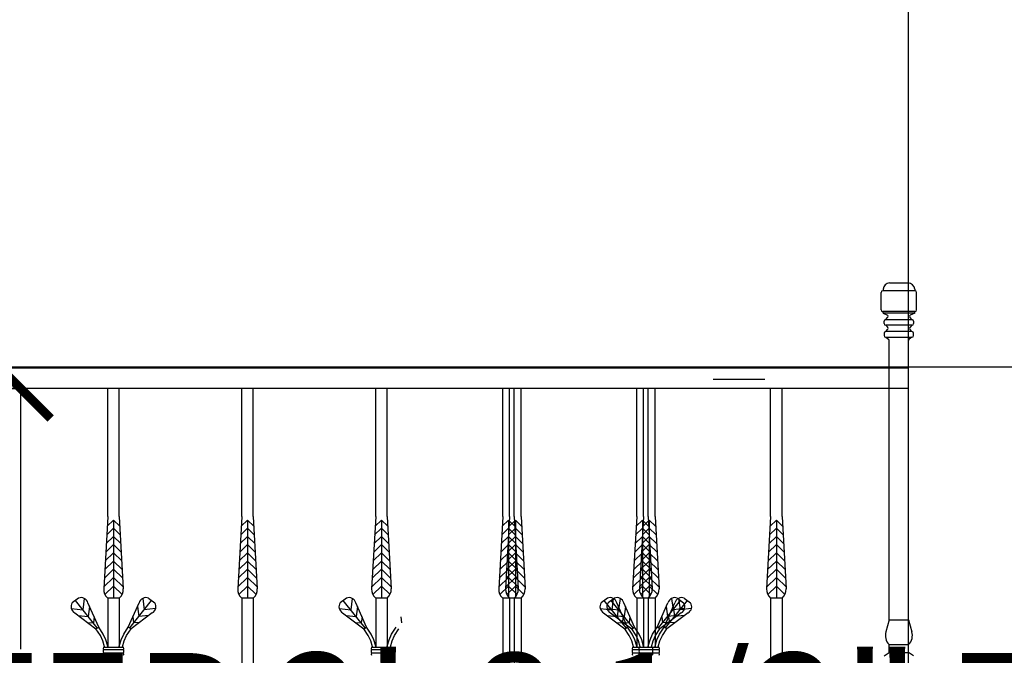
# Model space of a CAD drawing. Units: inches. Extents: x 2278 to 7495, y -71 to 1198.
# Tile 35 of 44: x 5101 to 5150, y 146 to 178. Entities that reach past the tile are written whole.
import ezdxf

# ---------------------------------------------------------------- set-up
doc = ezdxf.new("R2010")
doc.units = ezdxf.units.IN
doc.header["$MEASUREMENT"] = 0
doc.layers.add('A-ANNO-DIMS', color=2, linetype='Continuous', lineweight=18)
doc.layers.add('A-ELEV', color=7, linetype='Continuous', lineweight=25)
doc.styles.get("Standard").update_dxf_attribs({"font": 'arial.ttf'})
doc.dimstyles.get("Standard").update_dxf_attribs({"dimtxt": 6, "dimasz": 3, "dimexe": 0.18, "dimexo": 0.0625, "dimgap": 0.09, "dimtad": 0, "dimtih": 1, "dimtoh": 1, "dimdec": 0, "dimzin": 0, "dimdsep": 46, "dimlunit": 3, "dimtxsty": 'Standard', "dimblk": 'ARCHTICK', "dimcen": 0.09, "dimadec": 0, "dimazin": 0, "dimtfac": 1, "dimtdec": 0, "dimtofl": 0, "dimtmove": 0, "dimatfit": 3, "dimfxl": 1, "dimtolj": 1, "dimtzin": 0, "dimarcsym": 0})

# ---------------------------------------------------------------- blocks, each defined once
blk = doc.blocks.new('BALUSTER-ORNATE-A')
for p, q in [((3.585, 26.003), (3.585, 32.384)), ((4.155, 26.003), (4.155, 32.38)), ((3.585, 26.003), (3.383, 22.393)), ((3.558, 25.516), (3.87, 25.818)), ((3.87, 25.818), (3.87, 21.929)), ((4.182, 25.516), (3.87, 25.818)), ((4.155, 26.003), (4.357, 22.393)), ((3.533, 25.084), (3.87, 25.41)), ((4.207, 25.084), (3.87, 25.41)), ((3.485, 24.221), (3.87, 24.593)), ((3.509, 24.653), (3.87, 25.001)), ((4.231, 24.653), (3.87, 25.001)), ((4.255, 24.221), (3.87, 24.593)), ((3.461, 23.79), (3.87, 24.185)), ((4.279, 23.79), (3.87, 24.185)), ((3.437, 23.358), (3.87, 23.777)), ((4.303, 23.358), (3.87, 23.777)), ((3.413, 22.927), (3.87, 23.369)), ((4.327, 22.927), (3.87, 23.369)), ((3.388, 22.495), (3.87, 22.961)), ((4.352, 22.495), (3.87, 22.961)), ((3.442, 22.106), (3.87, 22.52)), ((4.299, 22.106), (3.87, 22.52)), ((2.128, 21.929), (1.813, 21.699)), ((3.063, 20.442), (1.97, 21.814)), ((2.412, 21.914), (2.339, 21.352)), ((3.131, 20.487), (2.594, 21.696)), ((3.585, 21.929), (3.585, 19.485)), ((4.155, 21.929), (3.585, 21.929)), ((4.155, 21.929), (4.155, 19.485)), ((4.609, 20.487), (5.146, 21.696)), ((4.677, 20.442), (5.77, 21.814)), ((5.328, 21.914), (5.401, 21.352)), ((5.612, 21.929), (5.927, 21.699)), ((1.774, 21.406), (2.339, 21.352)), ((1.936, 21.192), (2.995, 20.398)), ((2.678, 21.507), (2.613, 21.007)), ((5.804, 21.192), (4.745, 20.398)), ((5.062, 21.507), (5.127, 21.007)), ((5.966, 21.406), (5.401, 21.352)), ((2.111, 21.055), (2.613, 21.007)), ((2.562, 20.717), (2.868, 20.688)), ((2.907, 20.992), (2.868, 20.688)), ((4.833, 20.992), (4.872, 20.688)), ((5.178, 20.717), (4.872, 20.688)), ((5.629, 21.055), (5.127, 21.007)), ((2.995, 20.398), (3.131, 20.487)), ((3.217, 20.057), (2.995, 20.398)), ((3.36, 20.135), (3.131, 20.487)), ((3.49, 19.852), (3.36, 20.135)), ((4.25, 19.852), (4.38, 20.135)), ((4.38, 20.135), (4.609, 20.487)), ((4.523, 20.057), (4.745, 20.398)), ((4.745, 20.398), (4.609, 20.487)), ((3.337, 19.795), (3.217, 20.057)), ((3.421, 19.506), (3.337, 19.795)), ((3.585, 19.526), (3.49, 19.852)), ((4.155, 19.526), (4.25, 19.852)), ((4.319, 19.506), (4.403, 19.795)), ((4.403, 19.795), (4.523, 20.057)), ((3.37, 19.485), (4.37, 19.485)), ((3.37, 19.363), (4.37, 19.363)), ((3.37, 19.2), (4.37, 19.2)), ((3.42, 19.485), (3.421, 19.506)), ((3.583, 19.485), (3.585, 19.526)), ((4.157, 19.485), (4.155, 19.526)), ((4.32, 19.485), (4.319, 19.506))]:
    blk.add_line(p, q)
for centre, radius, start, end in [((3.929, 22.355), 0.547, 176.0178, 231.0717), ((3.811, 22.355), 0.547, 308.9283, 3.9822), ((2.111, 21.502), 0.356, 146.575, 240.6788), ((2.253, 21.595), 0.356, 16.4025, 110.5063), ((5.487, 21.595), 0.356, 69.4937, 163.5975), ((5.629, 21.502), 0.356, 299.3212, 33.425), ((3.475, 19.424), 0.121, 149.7768, 210.2232), ((3.563, 19.281), 0.209, 157.1017, 202.8983), ((3.475, 19.139), 0.121, 149.7768, 210.2232), ((4.265, 19.424), 0.121, 329.7768, 30.2232), ((4.177, 19.281), 0.209, 337.1017, 22.8983), ((4.265, 19.139), 0.121, 329.7768, 30.2232)]:
    blk.add_arc(centre, radius, start, end)
blk = doc.blocks.new('BALUSTER-ORNATE-B')
for p, q in [((3.585, 26.003), (3.585, 32.384)), ((4.155, 26.003), (4.155, 32.38)), ((3.585, 26.003), (3.383, 22.393)), ((3.558, 25.516), (3.87, 25.818)), ((3.87, 25.818), (3.87, 21.929)), ((4.183, 25.516), (3.87, 25.818)), ((4.155, 26.003), (4.358, 22.393)), ((3.534, 25.084), (3.87, 25.41)), ((4.207, 25.084), (3.87, 25.41)), ((3.485, 24.221), (3.87, 24.593)), ((3.51, 24.653), (3.87, 25.001)), ((4.231, 24.653), (3.87, 25.001)), ((4.255, 24.221), (3.87, 24.593)), ((3.461, 23.79), (3.87, 24.185)), ((4.279, 23.79), (3.87, 24.185)), ((3.437, 23.358), (3.87, 23.777)), ((4.304, 23.358), (3.87, 23.777)), ((3.413, 22.927), (3.87, 23.369)), ((4.328, 22.927), (3.87, 23.369)), ((3.389, 22.495), (3.87, 22.961)), ((4.352, 22.495), (3.87, 22.961)), ((3.442, 22.106), (3.87, 22.52)), ((4.299, 22.106), (3.87, 22.52)), ((2.128, 21.929), (1.814, 21.699)), ((3.063, 20.442), (1.971, 21.814)), ((2.412, 21.914), (2.339, 21.352)), ((3.132, 20.487), (2.595, 21.696)), ((3.585, 21.929), (3.585, 19.485)), ((4.155, 21.929), (3.585, 21.929)), ((4.155, 21.929), (4.155, 19.485)), ((1.774, 21.406), (2.339, 21.352)), ((1.936, 21.192), (2.995, 20.398)), ((2.679, 21.507), (2.614, 21.007)), ((2.112, 21.055), (2.614, 21.007)), ((2.563, 20.717), (2.868, 20.688)), ((2.907, 20.992), (2.868, 20.688)), ((4.833, 20.992), (4.873, 20.688)), ((2.995, 20.398), (3.132, 20.487)), ((3.217, 20.057), (2.995, 20.398)), ((3.36, 20.135), (3.132, 20.487)), ((3.49, 19.852), (3.36, 20.135)), ((4.251, 19.852), (4.381, 20.135)), ((4.381, 20.135), (4.609, 20.487)), ((4.524, 20.057), (4.746, 20.398)), ((3.337, 19.795), (3.217, 20.057)), ((3.421, 19.506), (3.337, 19.795)), ((3.585, 19.526), (3.49, 19.852)), ((4.155, 19.526), (4.251, 19.852)), ((4.319, 19.506), (4.404, 19.795)), ((4.404, 19.795), (4.524, 20.057)), ((3.37, 19.485), (4.37, 19.485)), ((3.37, 19.363), (4.37, 19.363)), ((3.37, 19.2), (4.37, 19.2)), ((3.42, 19.485), (3.421, 19.506)), ((3.583, 19.485), (3.585, 19.526)), ((4.157, 19.485), (4.155, 19.526)), ((4.32, 19.485), (4.319, 19.506))]:
    blk.add_line(p, q)
for centre, radius, start, end in [((3.929, 22.355), 0.547, 176.0178, 231.0717), ((3.811, 22.355), 0.547, 308.9283, 3.9822), ((2.111, 21.502), 0.356, 146.575, 240.6788), ((2.253, 21.595), 0.356, 16.4025, 110.5063), ((3.475, 19.424), 0.121, 149.7768, 210.2232), ((3.563, 19.281), 0.209, 157.1017, 202.8983), ((3.475, 19.139), 0.121, 149.7768, 210.2232), ((4.265, 19.424), 0.121, 329.7768, 30.2232), ((4.177, 19.281), 0.209, 337.1017, 22.8983), ((4.265, 19.139), 0.121, 329.7768, 30.2232)]:
    blk.add_arc(centre, radius, start, end)
blk = doc.blocks.new('RAIL-BAR-C')
for p, q in [((0.203, 26.003), (0.203, 32.38)), ((0.773, 32.38), (0.203, 32.38)), ((0.773, 26.003), (0.773, 32.38)), ((0.203, 26.003), (0, 22.393)), ((0.175, 25.516), (0.488, 25.818)), ((0.488, 25.818), (0.488, 21.929)), ((0.8, 25.516), (0.488, 25.818)), ((0.773, 26.003), (0.975, 22.393)), ((0.151, 25.084), (0.488, 25.41)), ((0.824, 25.084), (0.488, 25.41)), ((0.103, 24.221), (0.488, 24.593)), ((0.127, 24.653), (0.488, 25.001)), ((0.848, 24.653), (0.488, 25.001)), ((0.873, 24.221), (0.488, 24.593)), ((0.079, 23.79), (0.488, 24.185)), ((0.897, 23.79), (0.488, 24.185)), ((0.054, 23.358), (0.488, 23.777)), ((0.921, 23.358), (0.488, 23.777)), ((0.03, 22.927), (0.488, 23.369)), ((0.945, 22.927), (0.488, 23.369)), ((0.006, 22.495), (0.488, 22.961)), ((0.969, 22.495), (0.488, 22.961)), ((0.059, 22.106), (0.488, 22.52)), ((0.916, 22.106), (0.488, 22.52)), ((0.203, 21.929), (0.203, 7.128)), ((0.773, 21.929), (0.203, 21.929)), ((0.773, 21.929), (0.773, 7.128))]:
    blk.add_line(p, q)
for centre, start, end in [((0.547, 22.355), 176.0178, 231.0717), ((0.429, 22.355), 308.9283, 3.9822)]:
    blk.add_arc(centre, 0.547, start, end)
blk = doc.blocks.new('_ArchTick')
at = {"color": 0, "linetype": 'ByBlock', "const_width": 0.15}
blk.add_lwpolyline([(-0.5, -0.5), (0.5, 0.5)], dxfattribs=at)
blk = doc.blocks.new('*D59')
at = {"layer": 'A-ANNO-DIMS', "color": 0, "lineweight": -2, "transparency": 16777216}
for p, q in [((5096.589, 159.183), (5101.564, 159.183)), ((5101.384, 159.183), (5101.384, 146.185)), ((5101.384, 126.799), (5101.384, 139.796)), ((5096.589, 126.799), (5101.564, 126.799))]:
    blk.add_line(p, q, dxfattribs=at)
at = {"layer": 'Defpoints', "color": 0, "transparency": 16777216}
for p in [(5096.527, 159.183), (5101.384, 159.183), (5096.527, 126.799)]:
    blk.add_point(p, dxfattribs=at)
at = {"layer": 'A-ANNO-DIMS', "color": 0, "lineweight": -2, "transparency": 16777216, "xscale": 3, "yscale": 3, "zscale": 3}
for p, rotation in [((5101.384, 159.183), 90), ((5101.384, 126.799), 270)]:
    blk.add_blockref('_ArchTick', p, dxfattribs=dict(at, rotation=rotation))
at = {"layer": 'A-ANNO-DIMS', "color": 0, "transparency": 16777216, "insert": (5101.384, 142.991), "char_height": 6, "attachment_point": 5}
blk.add_mtext('\\A1;ORNATE BALUSTER 2\'-8 1/2" TYP.', dxfattribs=at)
blk = doc.blocks.new('*D123')
at = {"layer": 'A-ANNO-DIMS', "color": 0, "lineweight": -2, "transparency": 16777216}
for p, q in [((4736.95, 340.157), (4736.95, -23.427)), ((5145.676, -1.81), (5145.676, -23.427)), ((4736.95, -23.247), (4923.929, -23.247)), ((5145.676, -23.247), (4958.697, -23.247))]:
    blk.add_line(p, q, dxfattribs=at)
at = {"layer": 'Defpoints', "color": 0, "transparency": 16777216}
for p in [(4736.95, 340.219), (5145.676, -1.747), (5145.676, -23.247)]:
    blk.add_point(p, dxfattribs=at)
at = {"layer": 'A-ANNO-DIMS', "color": 0, "lineweight": -2, "transparency": 16777216, "xscale": 3, "yscale": 3, "zscale": 3, "rotation": 180}
blk.add_blockref('_ArchTick', (4736.95, -23.247), dxfattribs=at)
at = {"layer": 'A-ANNO-DIMS', "color": 0, "lineweight": -2, "transparency": 16777216, "xscale": 3, "yscale": 3, "zscale": 3}
blk.add_blockref('_ArchTick', (5145.676, -23.247), dxfattribs=at)
at = {"layer": 'A-ANNO-DIMS', "color": 0, "transparency": 16777216, "insert": (4941.313, -23.247), "char_height": 6, "attachment_point": 5}
blk.add_mtext('\\A1;34\'-0 1/2"', dxfattribs=at)
blk = doc.blocks.new('*D131')
at = {"layer": 'A-ANNO-DIMS', "color": 0, "lineweight": -2, "transparency": 16777216}
for p, q in [((5096.176, 99.315), (5096.176, 361.899)), ((5096.176, 361.719), (5105.75, 361.719)), ((5145.676, 361.719), (5136.102, 361.719)), ((5145.676, 118.315), (5145.676, 361.899))]:
    blk.add_line(p, q, dxfattribs=at)
at = {"layer": 'Defpoints', "color": 0, "transparency": 16777216}
for p in [(5145.676, 361.719), (5145.676, 118.253), (5096.176, 99.253)]:
    blk.add_point(p, dxfattribs=at)
at = {"layer": 'A-ANNO-DIMS', "color": 0, "lineweight": -2, "transparency": 16777216, "xscale": 3, "yscale": 3, "zscale": 3, "rotation": 180}
blk.add_blockref('_ArchTick', (5096.176, 361.719), dxfattribs=at)
at = {"layer": 'A-ANNO-DIMS', "color": 0, "lineweight": -2, "transparency": 16777216, "xscale": 3, "yscale": 3, "zscale": 3}
blk.add_blockref('_ArchTick', (5145.676, 361.719), dxfattribs=at)
at = {"layer": 'A-ANNO-DIMS', "color": 0, "transparency": 16777216, "insert": (5120.926, 361.719), "char_height": 6, "attachment_point": 5}
blk.add_mtext('\\A1;4\'-1 1/2"', dxfattribs=at)
blk = doc.blocks.new('*D139')
at = {"layer": 'A-ANNO-DIMS', "color": 0, "lineweight": -2, "transparency": 16777216}
for p, q in [((5092.239, 160.253), (5167.754, 160.253)), ((5167.574, 160.253), (5167.574, 142.408)), ((5167.574, 118.253), (5167.574, 136.097)), ((5145.739, 118.253), (5167.754, 118.253))]:
    blk.add_line(p, q, dxfattribs=at)
at = {"layer": 'Defpoints', "color": 0, "transparency": 16777216}
for p in [(5092.176, 160.253), (5167.574, 160.253), (5145.676, 118.253)]:
    blk.add_point(p, dxfattribs=at)
at = {"layer": 'A-ANNO-DIMS', "color": 0, "lineweight": -2, "transparency": 16777216, "xscale": 3, "yscale": 3, "zscale": 3}
for p, rotation in [((5167.574, 160.253), 90), ((5167.574, 118.253), 270)]:
    blk.add_blockref('_ArchTick', p, dxfattribs=dict(at, rotation=rotation))
at = {"layer": 'A-ANNO-DIMS', "color": 0, "transparency": 16777216, "insert": (5167.574, 139.253), "char_height": 6, "attachment_point": 5}
blk.add_mtext('\\A1;3\'-6"', dxfattribs=at)
blk = doc.blocks.new('*D140')
at = {"layer": 'A-ANNO-DIMS', "color": 0, "lineweight": -2, "transparency": 16777216}
for p, q in [((5096.239, 225.253), (5167.754, 225.253)), ((5167.574, 225.253), (5167.574, 195.894)), ((5167.574, 160.253), (5167.574, 189.612)), ((5092.239, 160.253), (5167.754, 160.253))]:
    blk.add_line(p, q, dxfattribs=at)
at = {"layer": 'Defpoints', "color": 0, "transparency": 16777216}
for p in [(5096.176, 225.253), (5167.574, 225.253), (5092.176, 160.253)]:
    blk.add_point(p, dxfattribs=at)
at = {"layer": 'A-ANNO-DIMS', "color": 0, "lineweight": -2, "transparency": 16777216, "xscale": 3, "yscale": 3, "zscale": 3}
for p, rotation in [((5167.574, 225.253), 90), ((5167.574, 160.253), 270)]:
    blk.add_blockref('_ArchTick', p, dxfattribs=dict(at, rotation=rotation))
at = {"layer": 'A-ANNO-DIMS', "color": 0, "transparency": 16777216, "insert": (5167.574, 192.753), "char_height": 6, "attachment_point": 5}
blk.add_mtext('\\A1;5\'-5"', dxfattribs=at)
blk = doc.blocks.new('*D144')
at = {"layer": 'A-ANNO-DIMS', "color": 0, "lineweight": -2, "transparency": 16777216}
for p, q in [((5145.739, 244.253), (5167.754, 244.253)), ((5167.574, 244.253), (5167.574, 184.406)), ((5167.574, 118.253), (5167.574, 178.099)), ((5145.739, 118.253), (5167.754, 118.253))]:
    blk.add_line(p, q, dxfattribs=at)
at = {"layer": 'Defpoints', "color": 0, "transparency": 16777216}
for p in [(5145.676, 244.253), (5167.574, 244.253), (5145.676, 118.253)]:
    blk.add_point(p, dxfattribs=at)
at = {"layer": 'A-ANNO-DIMS', "color": 0, "lineweight": -2, "transparency": 16777216, "xscale": 3, "yscale": 3, "zscale": 3}
for p, rotation in [((5167.574, 244.253), 90), ((5167.574, 118.253), 270)]:
    blk.add_blockref('_ArchTick', p, dxfattribs=dict(at, rotation=rotation))
at = {"layer": 'A-ANNO-DIMS', "color": 0, "transparency": 16777216, "insert": (5167.574, 181.253), "char_height": 6, "attachment_point": 5}
blk.add_mtext('\\A1;10\'-6"', dxfattribs=at)

msp = doc.modelspace()

# ---------------------------------------------------------------- linework, layer by layer
at = {"layer": 'A-ELEV'}
for p, q in [((5145.676, 164.446), (5145.676, 250.254)), ((5145.992, 164.046), (5144.383, 164.046)), ((5144.397, 164.122), (5144.397, 164.046)), ((5144.726, 164.449), (5145.648, 164.449)), ((5145.978, 164.122), (5145.978, 164.046)), ((5144.301, 163.092), (5144.301, 163.965)), ((5146.074, 163.092), (5146.074, 163.965)), ((5145.992, 163.01), (5144.383, 163.01)), ((5144.397, 162.934), (5144.397, 163.01)), ((5144.397, 162.934), (5144.622, 162.837)), ((5145.978, 162.934), (5144.397, 162.934)), ((5144.536, 162.615), (5144.622, 162.711)), ((5144.536, 162.615), (5145.839, 162.615)), ((5145.978, 162.934), (5145.753, 162.837)), ((5145.839, 162.615), (5145.753, 162.711)), ((5145.978, 162.934), (5145.978, 163.01)), ((5144.454, 162.416), (5144.454, 162.533)), ((5144.536, 162.334), (5144.622, 162.238)), ((5145.839, 162.334), (5144.536, 162.334)), ((5144.536, 162.015), (5144.622, 162.112)), ((5145.839, 162.334), (5145.753, 162.238)), ((5145.839, 162.015), (5145.753, 162.112)), ((5145.921, 162.533), (5145.921, 162.416)), ((5144.454, 161.934), (5144.454, 161.816)), ((5145.839, 162.015), (5144.536, 162.015)), ((5144.536, 161.735), (5144.669, 161.64)), ((5144.536, 161.735), (5145.839, 161.735)), ((5144.699, 147.642), (5144.699, 161.577)), ((5145.676, -1.747), (5145.676, 161.577)), ((5145.676, 147.642), (5145.676, 161.577)), ((5145.839, 161.735), (5145.706, 161.64)), ((5145.921, 161.816), (5145.921, 161.934)), ((5145.676, 160.198), (5066.016, 160.198)), ((5138.507, 159.631), (5135.918, 159.631)), ((5145.676, 159.179), (5066.016, 159.179)), ((5125.431, 152.802), (5125.431, 159.179)), ((5125.775, 152.802), (5125.775, 159.179)), ((5126.001, 152.802), (5126.001, 159.179)), ((5126.345, 152.802), (5126.345, 159.179)), ((5132.111, 152.802), (5132.111, 159.183)), ((5132.455, 152.802), (5132.455, 159.183)), ((5132.682, 152.802), (5132.682, 159.179)), ((5133.026, 152.802), (5133.026, 159.179)), ((5138.792, 152.802), (5138.792, 159.179)), ((5139.362, 152.802), (5139.362, 159.179)), ((5125.431, 152.802), (5125.229, 149.192)), ((5125.775, 152.802), (5125.573, 149.192)), ((5126.001, 152.802), (5126.203, 149.192)), ((5126.345, 152.802), (5126.547, 149.192)), ((5132.111, 152.802), (5131.909, 149.192)), ((5132.455, 152.802), (5132.253, 149.192)), ((5132.682, 152.802), (5132.884, 149.192)), ((5133.026, 152.802), (5133.228, 149.192)), ((5138.792, 152.802), (5138.59, 149.192)), ((5139.362, 152.802), (5139.564, 149.192)), ((5125.404, 152.315), (5125.716, 152.617)), ((5125.716, 152.617), (5125.716, 148.728)), ((5126.028, 152.315), (5125.716, 152.617)), ((5125.747, 152.315), (5126.06, 152.617)), ((5126.06, 152.617), (5126.06, 148.728)), ((5126.372, 152.315), (5126.06, 152.617)), ((5132.084, 152.315), (5132.397, 152.617)), ((5132.397, 152.617), (5132.397, 148.728)), ((5132.709, 152.315), (5132.397, 152.617)), ((5132.428, 152.315), (5132.74, 152.617)), ((5132.74, 152.617), (5132.74, 148.728)), ((5133.053, 152.315), (5132.74, 152.617)), ((5138.765, 152.315), (5139.077, 152.617)), ((5139.077, 152.617), (5139.077, 148.728)), ((5139.39, 152.315), (5139.077, 152.617)), ((5125.355, 151.452), (5125.716, 151.8)), ((5125.379, 151.883), (5125.716, 152.209)), ((5125.699, 151.452), (5126.06, 151.8)), ((5126.053, 151.883), (5125.716, 152.209)), ((5126.077, 151.452), (5125.716, 151.8)), ((5125.723, 151.883), (5126.06, 152.209)), ((5126.396, 151.883), (5126.06, 152.209)), ((5126.421, 151.452), (5126.06, 151.8)), ((5132.036, 151.452), (5132.397, 151.8)), ((5132.06, 151.883), (5132.397, 152.209)), ((5132.38, 151.452), (5132.74, 151.8)), ((5132.733, 151.883), (5132.397, 152.209)), ((5132.757, 151.452), (5132.397, 151.8)), ((5132.404, 151.883), (5132.74, 152.209)), ((5133.077, 151.883), (5132.74, 152.209)), ((5133.101, 151.452), (5132.74, 151.8)), ((5138.716, 151.452), (5139.077, 151.8)), ((5138.741, 151.883), (5139.077, 152.209)), ((5139.414, 151.883), (5139.077, 152.209)), ((5139.438, 151.452), (5139.077, 151.8)), ((5125.331, 151.02), (5125.716, 151.392)), ((5125.675, 151.02), (5126.06, 151.392)), ((5126.101, 151.02), (5125.716, 151.392)), ((5126.445, 151.02), (5126.06, 151.392)), ((5132.012, 151.02), (5132.397, 151.392)), ((5132.356, 151.02), (5132.74, 151.392)), ((5132.781, 151.02), (5132.397, 151.392)), ((5133.125, 151.02), (5132.74, 151.392)), ((5138.692, 151.02), (5139.077, 151.392)), ((5139.462, 151.02), (5139.077, 151.392)), ((5125.307, 150.589), (5125.716, 150.984)), ((5125.651, 150.589), (5126.06, 150.984)), ((5126.125, 150.589), (5125.716, 150.984)), ((5126.469, 150.589), (5126.06, 150.984)), ((5131.987, 150.589), (5132.397, 150.984)), ((5132.331, 150.589), (5132.74, 150.984)), ((5132.806, 150.589), (5132.397, 150.984)), ((5133.15, 150.589), (5132.74, 150.984)), ((5138.668, 150.589), (5139.077, 150.984)), ((5139.486, 150.589), (5139.077, 150.984)), ((5125.283, 150.157), (5125.716, 150.576)), ((5125.627, 150.157), (5126.06, 150.576)), ((5126.149, 150.157), (5125.716, 150.576)), ((5126.493, 150.157), (5126.06, 150.576)), ((5131.963, 150.157), (5132.397, 150.576)), ((5132.307, 150.157), (5132.74, 150.576)), ((5132.83, 150.157), (5132.397, 150.576)), ((5133.174, 150.157), (5132.74, 150.576)), ((5138.644, 150.157), (5139.077, 150.576)), ((5139.51, 150.157), (5139.077, 150.576)), ((5125.259, 149.726), (5125.716, 150.168)), ((5125.602, 149.726), (5126.06, 150.168)), ((5126.173, 149.726), (5125.716, 150.168)), ((5126.517, 149.726), (5126.06, 150.168)), ((5131.939, 149.726), (5132.397, 150.168)), ((5132.283, 149.726), (5132.74, 150.168)), ((5132.854, 149.726), (5132.397, 150.168)), ((5133.198, 149.726), (5132.74, 150.168)), ((5138.62, 149.726), (5139.077, 150.168)), ((5139.535, 149.726), (5139.077, 150.168)), ((5125.234, 149.294), (5125.716, 149.76)), ((5125.287, 148.905), (5125.716, 149.319)), ((5125.578, 149.294), (5126.06, 149.76)), ((5125.631, 148.905), (5126.06, 149.319)), ((5126.198, 149.294), (5125.716, 149.76)), ((5126.144, 148.905), (5125.716, 149.319)), ((5126.541, 149.294), (5126.06, 149.76)), ((5126.488, 148.905), (5126.06, 149.319)), ((5131.915, 149.294), (5132.397, 149.76)), ((5131.968, 148.905), (5132.397, 149.319)), ((5132.259, 149.294), (5132.74, 149.76)), ((5132.312, 148.905), (5132.74, 149.319)), ((5132.878, 149.294), (5132.397, 149.76)), ((5132.825, 148.905), (5132.397, 149.319)), ((5133.222, 149.294), (5132.74, 149.76)), ((5133.169, 148.905), (5132.74, 149.319)), ((5138.596, 149.294), (5139.077, 149.76)), ((5138.649, 148.905), (5139.077, 149.319)), ((5139.559, 149.294), (5139.077, 149.76)), ((5139.506, 148.905), (5139.077, 149.319)), ((5125.431, 148.728), (5125.431, 133.927)), ((5126.001, 148.728), (5125.431, 148.728)), ((5125.775, 148.728), (5125.775, 133.927)), ((5126.345, 148.728), (5125.775, 148.728)), ((5126.001, 148.728), (5126.001, 133.927)), ((5126.345, 148.728), (5126.345, 133.927)), ((5130.654, 148.728), (5130.34, 148.498)), ((5131.59, 147.241), (5130.497, 148.613)), ((5130.998, 148.728), (5130.684, 148.498)), ((5131.934, 147.241), (5130.841, 148.613)), ((5130.938, 148.713), (5130.865, 148.151)), ((5131.658, 147.286), (5131.121, 148.495)), ((5131.282, 148.713), (5131.209, 148.151)), ((5132.002, 147.286), (5131.465, 148.495)), ((5132.111, 148.728), (5132.111, 146.284)), ((5132.682, 148.728), (5132.111, 148.728)), ((5132.455, 148.728), (5132.455, 146.284)), ((5133.026, 148.728), (5132.455, 148.728)), ((5132.682, 148.728), (5132.682, 146.284)), ((5133.026, 148.728), (5133.026, 146.284)), ((5133.135, 147.286), (5133.672, 148.495)), ((5133.203, 147.241), (5134.296, 148.613)), ((5133.479, 147.286), (5134.016, 148.495)), ((5133.547, 147.241), (5134.64, 148.613)), ((5133.855, 148.713), (5133.928, 148.151)), ((5134.139, 148.728), (5134.453, 148.498)), ((5134.199, 148.713), (5134.272, 148.151)), ((5134.483, 148.728), (5134.797, 148.498)), ((5138.792, 148.728), (5138.792, 133.927)), ((5139.362, 148.728), (5138.792, 148.728)), ((5139.362, 148.728), (5139.362, 133.927)), ((5130.301, 148.205), (5130.865, 148.151)), ((5130.463, 147.991), (5131.521, 147.197)), ((5130.638, 147.854), (5131.14, 147.806)), ((5130.645, 148.205), (5131.209, 148.151)), ((5130.807, 147.991), (5131.865, 147.197)), ((5130.982, 147.854), (5131.484, 147.806)), ((5131.205, 148.306), (5131.14, 147.806)), ((5131.549, 148.306), (5131.484, 147.806)), ((5134.33, 147.991), (5133.272, 147.197)), ((5133.588, 148.306), (5133.653, 147.806)), ((5134.674, 147.991), (5133.616, 147.197)), ((5134.155, 147.854), (5133.653, 147.806)), ((5134.493, 148.205), (5133.928, 148.151)), ((5133.932, 148.306), (5133.997, 147.806)), ((5134.499, 147.854), (5133.997, 147.806)), ((5134.836, 148.205), (5134.272, 148.151)), ((5131.089, 147.516), (5131.394, 147.487)), ((5131.434, 147.791), (5131.394, 147.487)), ((5131.433, 147.516), (5131.738, 147.487)), ((5131.778, 147.791), (5131.738, 147.487)), ((5133.359, 147.791), (5133.399, 147.487)), ((5133.704, 147.516), (5133.399, 147.487)), ((5133.703, 147.791), (5133.743, 147.487)), ((5134.048, 147.516), (5133.743, 147.487)), ((5144.699, 147.642), (5144.546, 147.049)), ((5144.699, 147.642), (5145.676, 147.642)), ((5145.676, 147.642), (5145.829, 147.049)), ((5131.521, 147.197), (5131.658, 147.286)), ((5131.743, 146.856), (5131.521, 147.197)), ((5131.886, 146.934), (5131.658, 147.286)), ((5131.863, 146.594), (5131.743, 146.856)), ((5131.865, 147.197), (5132.002, 147.286)), ((5132.087, 146.856), (5131.865, 147.197)), ((5132.016, 146.651), (5131.886, 146.934)), ((5132.23, 146.934), (5132.002, 147.286)), ((5132.207, 146.594), (5132.087, 146.856)), ((5132.36, 146.651), (5132.23, 146.934)), ((5132.777, 146.651), (5132.907, 146.934)), ((5132.907, 146.934), (5133.135, 147.286)), ((5132.93, 146.594), (5133.05, 146.856)), ((5133.05, 146.856), (5133.272, 147.197)), ((5133.121, 146.651), (5133.251, 146.934)), ((5133.272, 147.197), (5133.135, 147.286)), ((5133.251, 146.934), (5133.479, 147.286)), ((5133.274, 146.594), (5133.394, 146.856)), ((5133.394, 146.856), (5133.616, 147.197)), ((5133.616, 147.197), (5133.479, 147.286)), ((5131.947, 146.305), (5131.863, 146.594)), ((5132.111, 146.325), (5132.016, 146.651)), ((5132.291, 146.305), (5132.207, 146.594)), ((5132.455, 146.325), (5132.36, 146.651)), ((5132.682, 146.325), (5132.777, 146.651)), ((5132.846, 146.305), (5132.93, 146.594)), ((5133.026, 146.325), (5133.121, 146.651)), ((5133.19, 146.305), (5133.274, 146.594)), ((5144.699, 146.42), (5145.676, 146.42)), ((5144.699, 146.012), (5144.699, 146.42)), ((5145.676, 146.012), (5145.676, 146.42)), ((5131.897, 146.284), (5132.897, 146.284)), ((5131.897, 146.162), (5132.897, 146.162)), ((5131.897, 145.999), (5132.897, 145.999)), ((5131.947, 146.284), (5131.947, 146.305)), ((5132.11, 146.284), (5132.111, 146.325)), ((5132.24, 146.284), (5133.241, 146.284)), ((5132.24, 146.162), (5133.241, 146.162)), ((5132.24, 145.999), (5133.241, 145.999)), ((5132.29, 146.284), (5132.291, 146.305)), ((5132.454, 146.284), (5132.455, 146.325)), ((5132.684, 146.284), (5132.682, 146.325)), ((5132.847, 146.284), (5132.846, 146.305)), ((5133.027, 146.284), (5133.026, 146.325)), ((5133.191, 146.284), (5133.19, 146.305)), ((5144.454, 145.849), (5144.699, 146.012)), ((5144.699, 146.012), (5145.676, 146.012)), ((5145.921, 145.849), (5145.676, 146.012))]:
    msp.add_line(p, q, dxfattribs=at)
for centre, radius, start, end in [((5144.383, 163.965), 0.0815, 90, 180), ((5144.749, 164.097), 0.352, 93.6206, 175.8919), ((5145.626, 164.097), 0.352, 4.1081, 86.3794), ((5145.992, 163.965), 0.0815, 0, 90), ((5144.383, 163.092), 0.0815, 180, 270), ((5145.992, 163.092), 0.0815, 270, 0), ((5144.536, 162.533), 0.0815, 90, 180), ((5144.57, 162.774), 0.0815, 309.328, 50.672), ((5145.805, 162.774), 0.0815, 129.328, 230.672), ((5145.839, 162.533), 0.0815, 0, 90), ((5144.536, 162.416), 0.0815, 180, 270), ((5144.57, 162.175), 0.0815, 309.328, 50.672), ((5145.805, 162.175), 0.0815, 129.328, 230.672), ((5145.839, 162.416), 0.0815, 270, 360), ((5144.536, 161.934), 0.0815, 90, 180), ((5144.536, 161.816), 0.0815, 180, 270), ((5144.617, 161.577), 0.0815, 0, 50.672), ((5145.758, 161.577), 0.0815, 129.328, 180), ((5145.839, 161.934), 0.0815, 0, 90), ((5145.839, 161.816), 0.0815, 270, 360), ((5125.775, 149.154), 0.547, 176.0178, 231.0717), ((5126.119, 149.154), 0.547, 176.0178, 231.0717), ((5125.657, 149.154), 0.547, 308.9283, 3.9822), ((5126.001, 149.154), 0.547, 308.9283, 3.9822), ((5132.455, 149.154), 0.547, 176.0178, 231.0717), ((5132.799, 149.154), 0.547, 176.0178, 231.0717), ((5132.338, 149.154), 0.547, 308.9283, 3.9822), ((5132.682, 149.154), 0.547, 308.9283, 3.9822), ((5139.136, 149.154), 0.547, 176.0178, 231.0717), ((5139.018, 149.154), 0.547, 308.9283, 3.9822), ((5130.637, 148.301), 0.356, 146.575, 240.6788), ((5130.981, 148.301), 0.356, 146.575, 240.6788), ((5130.779, 148.394), 0.356, 16.4025, 110.5063), ((5131.123, 148.394), 0.356, 16.4025, 110.5063), ((5134.014, 148.394), 0.356, 69.4937, 163.5975), ((5134.358, 148.394), 0.356, 69.4937, 163.5975), ((5134.156, 148.301), 0.356, 299.3212, 33.425), ((5134.5, 148.301), 0.356, 299.3212, 33.425), ((5145.122, 146.856), 0.608, 161.4732, 225.8681), ((5145.253, 146.856), 0.608, 314.1319, 18.5268), ((5132.001, 146.223), 0.121, 149.7768, 210.2232), ((5132.089, 146.08), 0.209, 157.1017, 202.8983), ((5132.001, 145.938), 0.121, 149.7768, 210.2232), ((5132.345, 146.223), 0.121, 149.7768, 210.2232), ((5132.433, 146.08), 0.209, 157.1017, 202.8983), ((5132.345, 145.938), 0.121, 149.7768, 210.2232), ((5132.792, 146.223), 0.121, 329.7768, 30.2232), ((5132.704, 146.08), 0.209, 337.1017, 22.8983), ((5132.792, 145.938), 0.121, 329.7768, 30.2232), ((5133.136, 146.223), 0.121, 329.7768, 30.2232), ((5133.048, 146.08), 0.209, 337.1017, 22.8983), ((5133.136, 145.938), 0.121, 329.7768, 30.2232)]:
    msp.add_arc(centre, radius, start, end, dxfattribs=at)

# ---------------------------------------------------------------- block references
for name, p in [('BALUSTER-ORNATE-A', (5102.148, 126.799)), ('RAIL-BAR-C', (5112.211, 126.799)), ('BALUSTER-ORNATE-B', (5115.509, 126.799))]:
    msp.add_blockref(name, p, dxfattribs=at)

# ---------------------------------------------------------------- dimensions: what is measured, and where the dimension line sits
at = {"layer": 'A-ANNO-DIMS'}
for base, p1, p2, picture, middle in [((5145.676, 361.719), (5096.176, 99.253), (5145.676, 118.253), '*D131', (5120.926, 361.719)), ((5145.676, -23.247), (4736.95, 340.219), (5145.676, -1.747), '*D123', (4941.313, -23.247))]:
    dim = msp.add_linear_dim(base=base, p1=p1, p2=p2, dimstyle='Standard', override={"dimdec": 1, "dimlfac": 1, "dimrnd": 0, "dimzin": 1, "dimdsep": 46, "dimlunit": 4, "dimfrac": 2}, dxfattribs=at)
    dim.commit()
    dim.dimension.update_dxf_attribs({"geometry": picture, "text_midpoint": middle})
for base, p1, p2, picture, middle in [((5167.574, 244.253), (5145.676, 118.253), (5145.676, 244.253), '*D144', (5167.574, 181.253)), ((5167.574, 225.253), (5092.176, 160.253), (5096.176, 225.253), '*D140', (5167.574, 192.753)), ((5167.574, 160.253), (5145.676, 118.253), (5092.176, 160.253), '*D139', (5167.574, 139.253))]:
    dim = msp.add_linear_dim(base=base, p1=p1, p2=p2, angle=90, dimstyle='Standard', override={"dimdec": 1, "dimlfac": 1, "dimrnd": 0, "dimzin": 1, "dimdsep": 46, "dimlunit": 4, "dimfrac": 2}, dxfattribs=at)
    dim.commit()
    dim.dimension.update_dxf_attribs({"geometry": picture, "text_midpoint": middle})
dim = msp.add_linear_dim(base=(5101.384, 159.183), p1=(5096.527, 126.799), p2=(5096.527, 159.183), angle=90, text='ORNATE BALUSTER <> TYP.', dimstyle='Standard', override={"dimdec": 1, "dimrnd": 0, "dimzin": 1, "dimlunit": 4, "dimfrac": 2}, dxfattribs=at)
dim.commit()
dim.dimension.update_dxf_attribs({"geometry": '*D59', "text_midpoint": (5101.384, 142.991)})

doc.saveas('drawing.dxf')
